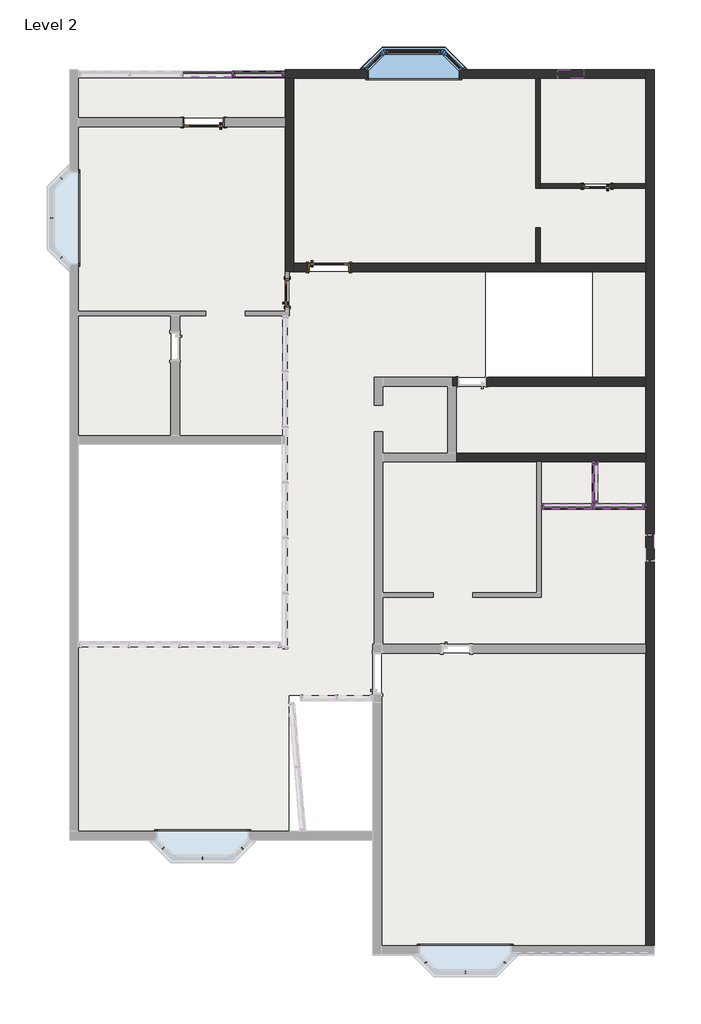
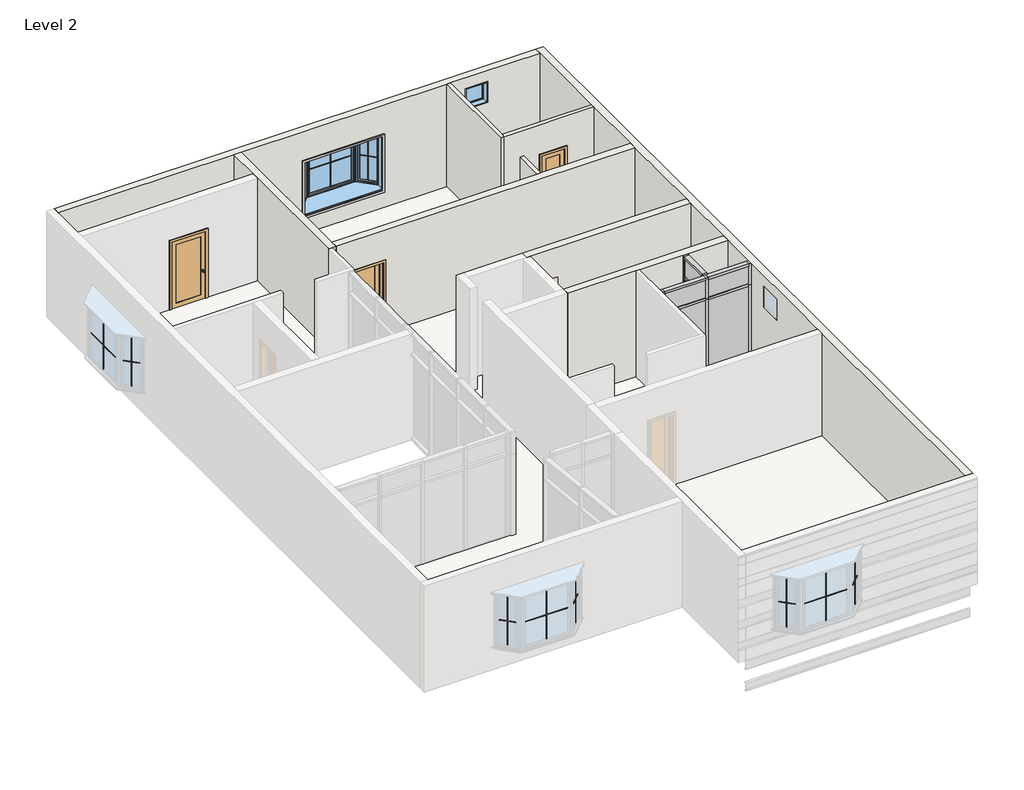
# One storey, part 5 of 5: 24 members, 16 proxies, 9 walls, 8 plates, 4 doors, 3 slabs, 2 windows.
"""IFC4 building model written with IfcOpenShell, lengths in millimetres."""

from ifc_helpers import new_model, si_unit, frame, origin, place, context, project, spatial, polyline, outline, extrude, faceted_brep, transform, mapped, element, save
from components import muntin_pattern_2x2_muntin_pattern_2x2_511ed329, muntin_pattern_2x2_muntin_pattern_2x2_63bd3b25, trim_window_interior_flat_picture_frame_e25f2530, door_interior_single_1_panel_wood_33af59b7, door_82825f5f, door_interior_single_1_panel_wood_secondary_door_3_x_7_9c4ddfbd, member_6e77e263, member_47bfaf8a, member_aaf6ec4e, member_7ce6cacc, member_f0fea5a5, member_ee409385, member_86adc6a2, member_92f44db0, member_11eb1482, member_fb055d8d, member_66f4a397, member_e9262278, system_panel_glazed_37c910ec, system_panel_glazed_3c79bf9a, system_panel_glazed_51086eaf, system_panel_glazed_73486e20, system_panel_glazed_4fbe648e, system_panel_glazed_a20b732f, window_6846e476, window_9f89e8e4

model = new_model("IFC4")

# Units and contexts
model_context = context("Model", 3, world=origin())
ifc_project = project(units=[si_unit("LENGTHUNIT", "METRE", prefix="MILLI")], contexts=[model_context])

# Site, building, storey
site = spatial("IfcSite", under=ifc_project)
building = spatial("IfcBuilding", under=site)
storey = spatial("IfcBuildingStorey", under=building, Name="Level 2", Elevation=3048.0)

# Proxies
placement = place(None, origin())
muntin_pattern_2x2_muntin_pattern_2x2_shape = muntin_pattern_2x2_muntin_pattern_2x2_511ed329(model_context)
element("IfcBuildingElementProxy", 1, Name="Muntin Pattern_2x2 : Muntin Pattern_2x2", ObjectType="Muntin Pattern_2x2 : Muntin Pattern_2x2", at=placement, inside=storey, context=model_context, shape_type="MappedRepresentation", body=[
    mapped(muntin_pattern_2x2_muntin_pattern_2x2_shape, transform((-41615.3380314, -10417.0163973, 3778.25), x_axis=(-1.0, 0.0, 0.0), y_axis=(0.0, -1.0, 0.0), z_axis=(0.0, 0.0, 1.0))),
])
element("IfcBuildingElementProxy", 2, Name="Muntin Pattern_2x2 : Muntin Pattern_2x2", ObjectType="Muntin Pattern_2x2 : Muntin Pattern_2x2", at=placement, inside=storey, context=model_context, shape_type="MappedRepresentation", body=[
    mapped(muntin_pattern_2x2_muntin_pattern_2x2_shape, transform((-42809.1380314, 10861.8336027, 3778.25), x_axis=(1.0, 0.0, 0.0), y_axis=(0.0, 1.0, 0.0), z_axis=(0.0, 0.0, 1.0))),
])
element("IfcBuildingElementProxy", 3, Name="Muntin Pattern_2x2 : Muntin Pattern_2x2", ObjectType="Muntin Pattern_2x2 : Muntin Pattern_2x2", at=placement, inside=storey, context=model_context, shape_type="MappedRepresentation", body=[
    mapped(muntin_pattern_2x2_muntin_pattern_2x2_shape, transform((-51175.2630314, 7016.9086027, 3778.25), x_axis=(0.0, 1.0, 0.0), y_axis=(-1.0, 0.0, 0.0), z_axis=(0.0, 0.0, 1.0))),
])
element("IfcBuildingElementProxy", 4, Name="Muntin Pattern_2x2 : Muntin Pattern_2x2", ObjectType="Muntin Pattern_2x2 : Muntin Pattern_2x2", at=placement, inside=storey, context=model_context, shape_type="MappedRepresentation", body=[
    mapped(muntin_pattern_2x2_muntin_pattern_2x2_shape, transform((-47685.9380314, -7775.4163973, 3778.25), x_axis=(-1.0, 0.0, 0.0), y_axis=(0.0, -1.0, 0.0), z_axis=(0.0, 0.0, 1.0))),
])
muntin_pattern_2x2_muntin_pattern_2x2_2_shape = muntin_pattern_2x2_muntin_pattern_2x2_63bd3b25(model_context)
element("IfcBuildingElementProxy", 5, Name="Muntin Pattern_2x2 : Muntin Pattern_2x2", ObjectType="Muntin Pattern_2x2 : Muntin Pattern_2x2", at=placement, inside=storey, context=model_context, shape_type="MappedRepresentation", body=[
    mapped(muntin_pattern_2x2_muntin_pattern_2x2_2_shape, transform((-40700.6463026, -10189.1206929, 3778.25), x_axis=(-0.7071067811865506, -0.7071067811865447, 0.0), y_axis=(0.7071067811865447, -0.7071067811865506, 0.0), z_axis=(0.0, 0.0, 1.0))),
])
element("IfcBuildingElementProxy", 6, Name="Muntin Pattern_2x2 : Muntin Pattern_2x2", ObjectType="Muntin Pattern_2x2 : Muntin Pattern_2x2", at=placement, inside=storey, context=model_context, shape_type="MappedRepresentation", body=[
    mapped(muntin_pattern_2x2_muntin_pattern_2x2_2_shape, transform((-42530.0297602, -10189.1206929, 3778.25), x_axis=(-0.7071067811865459, 0.7071067811865492, 0.0), y_axis=(-0.7071067811865492, -0.7071067811865459, 0.0), z_axis=(0.0, 0.0, 1.0))),
])
element("IfcBuildingElementProxy", 7, Name="Muntin Pattern_2x2 : Muntin Pattern_2x2", ObjectType="Muntin Pattern_2x2 : Muntin Pattern_2x2", at=placement, inside=storey, context=model_context, shape_type="MappedRepresentation", body=[
    mapped(muntin_pattern_2x2_muntin_pattern_2x2_2_shape, transform((-43723.8297602, 10633.9378984, 3778.25), x_axis=(0.7071067811865505, 0.7071067811865448, 0.0), y_axis=(-0.7071067811865448, 0.7071067811865505, 0.0), z_axis=(0.0, 0.0, 1.0))),
])
element("IfcBuildingElementProxy", 8, Name="Muntin Pattern_2x2 : Muntin Pattern_2x2", ObjectType="Muntin Pattern_2x2 : Muntin Pattern_2x2", at=placement, inside=storey, context=model_context, shape_type="MappedRepresentation", body=[
    mapped(muntin_pattern_2x2_muntin_pattern_2x2_2_shape, transform((-41894.4463026, 10633.9378984, 3778.25), x_axis=(0.707106781186546, -0.7071067811865491, 0.0), y_axis=(0.7071067811865491, 0.707106781186546, 0.0), z_axis=(0.0, 0.0, 1.0))),
])
element("IfcBuildingElementProxy", 9, Name="Muntin Pattern_2x2 : Muntin Pattern_2x2", ObjectType="Muntin Pattern_2x2 : Muntin Pattern_2x2", at=placement, inside=storey, context=model_context, shape_type="MappedRepresentation", body=[
    mapped(muntin_pattern_2x2_muntin_pattern_2x2_2_shape, transform((-50947.3673271, 6102.2168739, 3778.25), x_axis=(-0.707106781186546, 0.7071067811865492, 0.0), y_axis=(-0.7071067811865492, -0.707106781186546, 0.0), z_axis=(0.0, 0.0, 1.0))),
])
element("IfcBuildingElementProxy", 10, Name="Muntin Pattern_2x2 : Muntin Pattern_2x2", ObjectType="Muntin Pattern_2x2 : Muntin Pattern_2x2", at=placement, inside=storey, context=model_context, shape_type="MappedRepresentation", body=[
    mapped(muntin_pattern_2x2_muntin_pattern_2x2_2_shape, transform((-50947.3673271, 7931.6003316, 3778.25), x_axis=(0.7071067811865479, 0.7071067811865472, 0.0), y_axis=(-0.7071067811865472, 0.7071067811865479, 0.0), z_axis=(0.0, 0.0, 1.0))),
])
element("IfcBuildingElementProxy", 11, Name="Muntin Pattern_2x2 : Muntin Pattern_2x2", ObjectType="Muntin Pattern_2x2 : Muntin Pattern_2x2", at=placement, inside=storey, context=model_context, shape_type="MappedRepresentation", body=[
    mapped(muntin_pattern_2x2_muntin_pattern_2x2_2_shape, transform((-46771.2463026, -7547.5206929, 3778.25), x_axis=(-0.7071067811865506, -0.7071067811865447, 0.0), y_axis=(0.7071067811865447, -0.7071067811865506, 0.0), z_axis=(0.0, 0.0, 1.0))),
])
element("IfcBuildingElementProxy", 12, Name="Muntin Pattern_2x2 : Muntin Pattern_2x2", ObjectType="Muntin Pattern_2x2 : Muntin Pattern_2x2", at=placement, inside=storey, context=model_context, shape_type="MappedRepresentation", body=[
    mapped(muntin_pattern_2x2_muntin_pattern_2x2_2_shape, transform((-48600.6297602, -7547.5206929, 3778.25), x_axis=(-0.7071067811865459, 0.7071067811865492, 0.0), y_axis=(-0.7071067811865492, -0.7071067811865459, 0.0), z_axis=(0.0, 0.0, 1.0))),
])
trim_window_interior_flat_picture_frame_shape = trim_window_interior_flat_picture_frame_e25f2530(model_context)
element("IfcBuildingElementProxy", 13, Name="Trim-Window-Interior-Flat : Picture Frame", ObjectType="Trim-Window-Interior-Flat : Picture Frame", at=placement, inside=storey, context=model_context, shape_type="MappedRepresentation", body=[
    mapped(trim_window_interior_flat_picture_frame_shape, transform((-41615.3380314, -9797.8913973, 5232.4), x_axis=(-1.0, 0.0, 0.0), y_axis=(0.0, 0.0, 1.0), z_axis=(0.0, 1.0, 0.0))),
])
element("IfcBuildingElementProxy", 14, Name="Trim-Window-Interior-Flat : Picture Frame", ObjectType="Trim-Window-Interior-Flat : Picture Frame", at=placement, inside=storey, context=model_context, shape_type="MappedRepresentation", body=[
    mapped(trim_window_interior_flat_picture_frame_shape, transform((-42809.1380314, 10242.7086027, 5232.4), x_axis=(1.0, 0.0, 0.0), y_axis=(0.0, 0.0, 1.0), z_axis=(0.0, -1.0, 0.0))),
])
element("IfcBuildingElementProxy", 15, Name="Trim-Window-Interior-Flat : Picture Frame", ObjectType="Trim-Window-Interior-Flat : Picture Frame", at=placement, inside=storey, context=model_context, shape_type="MappedRepresentation", body=[
    mapped(trim_window_interior_flat_picture_frame_shape, transform((-50556.1380314, 7016.9086027, 5232.4), x_axis=(0.0, 1.0, 0.0), y_axis=(0.0, 0.0, 1.0), z_axis=(1.0, 0.0, 0.0))),
])
element("IfcBuildingElementProxy", 16, Name="Trim-Window-Interior-Flat : Picture Frame", ObjectType="Trim-Window-Interior-Flat : Picture Frame", at=placement, inside=storey, context=model_context, shape_type="MappedRepresentation", body=[
    mapped(trim_window_interior_flat_picture_frame_shape, transform((-47685.9380314, -7156.2913973, 5232.4), x_axis=(-1.0, 0.0, 0.0), y_axis=(0.0, 0.0, 1.0), z_axis=(0.0, 1.0, 0.0))),
])

# Doors
door_interior_single_1_panel_wood_shape = door_interior_single_1_panel_wood_33af59b7(model_context)
element("IfcDoor", 17, ObjectType="Door-Interior-Single-1_Panel-Wood", at=placement, inside=storey, context=model_context, shape_type="MappedRepresentation", body=[
    mapped(door_interior_single_1_panel_wood_shape, transform((-45733.3130314, 5289.7086027, 3048.0), x_axis=(0.0, 1.0, 0.0), y_axis=(-1.0, 0.0, 0.0), z_axis=(0.0, 0.0, 1.0))),
])
element("IfcDoor", 18, ObjectType="Door-Interior-Single-1_Panel-Wood", at=placement, inside=storey, context=model_context, shape_type="MappedRepresentation", body=[
    mapped(door_interior_single_1_panel_wood_shape, transform((-38567.3380314, 7750.3336027, 3048.0), x_axis=(-1.0, 0.0, 0.0), y_axis=(0.0, -1.0, 0.0), z_axis=(0.0, 0.0, 1.0))),
])
door_shape = door_82825f5f(model_context)
element("IfcDoor", 19, ObjectType="Door-Interior-Single-1_Panel-Wood : 36\" x 80\"", at=placement, inside=storey, context=model_context, shape_type="MappedRepresentation", body=[
    mapped(door_shape, transform((-47660.5380314, 9223.5336027, 3048.0), x_axis=(-1.0, 0.0, 0.0), y_axis=(0.0, -1.0, 0.0), z_axis=(0.0, 0.0, 1.0))),
])
door_interior_single_1_panel_wood_secondary_door_3_x_7_shape = door_interior_single_1_panel_wood_secondary_door_3_x_7_9c4ddfbd(model_context)
element("IfcDoor", 20, ObjectType="Door-Interior-Single-1_Panel-Wood : SECONDARY DOOR 3' X 7'", at=placement, inside=storey, context=model_context, shape_type="MappedRepresentation", body=[
    mapped(door_interior_single_1_panel_wood_secondary_door_3_x_7_shape, transform((-44764.9380314, 5877.0836027, 3048.0), x_axis=(1.0, 0.0, 0.0), y_axis=(0.0, 1.0, 0.0), z_axis=(0.0, 0.0, 1.0))),
])

# Members
member_shape = member_6e77e263(model_context)
element("IfcMember", 21, ObjectType="Rectangular Mullion : 2.5\" x 5\" rectangular", at=placement, inside=storey, context=model_context, shape_type="MappedRepresentation", body=[
    mapped(member_shape, transform((-38656.2380314, 354.3957124, 5486.4), x_axis=(1.0, 0.0, 0.0), y_axis=(0.0, -1.0, 0.0), z_axis=(0.0, 0.0, -1.0))),
])
member_2_shape = member_47bfaf8a(model_context)
element("IfcMember", 22, ObjectType="Rectangular Mullion : 2.5\" x 5\" rectangular", at=placement, inside=storey, context=model_context, shape_type="MappedRepresentation", body=[
    mapped(member_2_shape, transform((-39862.7380314, 354.3957124, 6096.0), x_axis=(-1.0, 0.0, 0.0), y_axis=(0.0, -1.0, 0.0), z_axis=(0.0, 0.0, 1.0))),
])
element("IfcMember", 23, ObjectType="Rectangular Mullion : 2.5\" x 5\" rectangular", at=placement, inside=storey, context=model_context, shape_type="MappedRepresentation", body=[
    mapped(member_2_shape, transform((-37449.7380314, 354.3957124, 5486.4), x_axis=(1.0, 0.0, 0.0), y_axis=(0.0, -1.0, 0.0), z_axis=(0.0, 0.0, -1.0))),
])
member_3_shape = member_aaf6ec4e(model_context)
element("IfcMember", 24, ObjectType="Rectangular Mullion : 2.5\" x 5\" rectangular", at=placement, inside=storey, context=model_context, shape_type="MappedRepresentation", body=[
    mapped(member_3_shape, transform((-37513.2380314, 354.3957124, 6096.0), x_axis=(0.0, 0.0, 1.0), y_axis=(0.0, -1.0, 0.0), z_axis=(1.0, 0.0, 0.0))),
])
element("IfcMember", 25, ObjectType="Rectangular Mullion : 2.5\" x 5\" rectangular", at=placement, inside=storey, context=model_context, shape_type="MappedRepresentation", body=[
    mapped(member_3_shape, transform((-38687.9880314, 354.3957124, 6096.0), x_axis=(0.0, 0.0, 1.0), y_axis=(0.0, -1.0, 0.0), z_axis=(1.0, 0.0, 0.0))),
])
element("IfcMember", 26, ObjectType="Rectangular Mullion : 2.5\" x 5\" rectangular", at=placement, inside=storey, context=model_context, shape_type="MappedRepresentation", body=[
    mapped(member_3_shape, transform((-39799.2380314, 354.3957124, 3048.0), x_axis=(0.0, 0.0, -1.0), y_axis=(0.0, -1.0, 0.0), z_axis=(-1.0, 0.0, 0.0))),
])
element("IfcMember", 27, ObjectType="Rectangular Mullion : 2.5\" x 5\" rectangular", at=placement, inside=storey, context=model_context, shape_type="MappedRepresentation", body=[
    mapped(member_3_shape, transform((-38624.4880314, 354.3957124, 3048.0), x_axis=(0.0, 0.0, -1.0), y_axis=(0.0, -1.0, 0.0), z_axis=(-1.0, 0.0, 0.0))),
])
member_4_shape = member_7ce6cacc(model_context)
element("IfcMember", 28, ObjectType="Rectangular Mullion : 2.5\" x 5\" rectangular", at=placement, inside=storey, context=model_context, shape_type="MappedRepresentation", body=[
    mapped(member_4_shape, transform((-38687.9880314, 354.3957124, 5486.4), x_axis=(0.0, 0.0, 1.0), y_axis=(0.0, -1.0, 0.0), z_axis=(1.0, 0.0, 0.0))),
])
element("IfcMember", 29, ObjectType="Rectangular Mullion : 2.5\" x 5\" rectangular", at=placement, inside=storey, context=model_context, shape_type="MappedRepresentation", body=[
    mapped(member_4_shape, transform((-37513.2380314, 354.3957124, 5486.4), x_axis=(0.0, 0.0, 1.0), y_axis=(0.0, -1.0, 0.0), z_axis=(1.0, 0.0, 0.0))),
])
member_5_shape = member_f0fea5a5(model_context)
element("IfcMember", 30, ObjectType="Rectangular Mullion : 2.5\" x 5\" rectangular", at=placement, inside=storey, context=model_context, shape_type="MappedRepresentation", body=[
    mapped(member_5_shape, transform((-38656.2380314, 354.3957124, 3048.0), x_axis=(1.0, 0.0, 0.0), y_axis=(0.0, -1.0, 0.0), z_axis=(0.0, 0.0, -1.0))),
])
member_6_shape = member_ee409385(model_context)
element("IfcMember", 31, ObjectType="Rectangular Mullion : 2.5\" x 5\" rectangular", at=placement, inside=storey, context=model_context, shape_type="MappedRepresentation", body=[
    mapped(member_6_shape, transform((-37449.7380314, 354.3957124, 3048.0), x_axis=(1.0, 0.0, 0.0), y_axis=(0.0, -1.0, 0.0), z_axis=(0.0, 0.0, -1.0))),
])
element("IfcMember", 32, ObjectType="Rectangular Mullion : 2.5\" x 5\" rectangular", at=placement, inside=storey, context=model_context, shape_type="MappedRepresentation", body=[
    mapped(member_6_shape, transform((-39862.7380314, 354.3957124, 5486.4), x_axis=(-1.0, 0.0, 0.0), y_axis=(0.0, -1.0, 0.0), z_axis=(0.0, 0.0, 1.0))),
])
element("IfcMember", 33, ObjectType="Rectangular Mullion : 2.5\" x 5\" rectangular", at=placement, inside=storey, context=model_context, shape_type="MappedRepresentation", body=[
    mapped(member_6_shape, transform((-38618.1380314, 1378.1086027, 3048.0), x_axis=(0.0, 1.0, 0.0), y_axis=(1.0, 0.0, 0.0), z_axis=(0.0, 0.0, -1.0))),
])
element("IfcMember", 34, ObjectType="Rectangular Mullion : 2.5\" x 5\" rectangular", at=placement, inside=storey, context=model_context, shape_type="MappedRepresentation", body=[
    mapped(member_2_shape, transform((-38618.1380314, 412.9086027, 6096.0), x_axis=(0.0, -1.0, 0.0), y_axis=(1.0, 0.0, 0.0), z_axis=(0.0, 0.0, 1.0))),
])
element("IfcMember", 35, ObjectType="Rectangular Mullion : 2.5\" x 5\" rectangular", at=placement, inside=storey, context=model_context, shape_type="MappedRepresentation", body=[
    mapped(member_2_shape, transform((-38618.1380314, 1378.1086027, 5486.4), x_axis=(0.0, 1.0, 0.0), y_axis=(1.0, 0.0, 0.0), z_axis=(0.0, 0.0, -1.0))),
])
element("IfcMember", 36, ObjectType="Rectangular Mullion : 2.5\" x 5\" rectangular", at=placement, inside=storey, context=model_context, shape_type="MappedRepresentation", body=[
    mapped(member_6_shape, transform((-38618.1380314, 412.9086027, 5486.4), x_axis=(0.0, -1.0, 0.0), y_axis=(1.0, 0.0, 0.0), z_axis=(0.0, 0.0, 1.0))),
])
member_7_shape = member_86adc6a2(model_context)
element("IfcMember", 37, ObjectType="Rectangular Mullion : 2.5\" x 5\" rectangular", at=placement, inside=storey, context=model_context, shape_type="MappedRepresentation", body=[
    mapped(member_7_shape, transform((-38618.1380314, 1314.6086027, 6096.0), x_axis=(0.0, 0.0, 1.0), y_axis=(1.0, 0.0, 0.0), z_axis=(0.0, 1.0, 0.0))),
])
element("IfcMember", 38, ObjectType="Rectangular Mullion : 2.5\" x 5\" rectangular", at=placement, inside=storey, context=model_context, shape_type="MappedRepresentation", body=[
    mapped(member_7_shape, transform((-38618.1380314, 476.4086027, 3048.0), x_axis=(0.0, 0.0, -1.0), y_axis=(1.0, 0.0, 0.0), z_axis=(0.0, -1.0, 0.0))),
])
member_8_shape = member_92f44db0(model_context)
element("IfcMember", 39, ObjectType="Rectangular Mullion : 2.5\" x 5\" rectangular", at=placement, inside=storey, context=model_context, shape_type="MappedRepresentation", body=[
    mapped(member_8_shape, transform((-38618.1380314, 1314.6086027, 5486.4), x_axis=(0.0, 0.0, 1.0), y_axis=(1.0, 0.0, 0.0), z_axis=(0.0, 1.0, 0.0))),
])
member_9_shape = member_11eb1482(model_context)
element("IfcMember", 40, ObjectType="Rectangular Mullion : 2.5\" x 5\" rectangular", at=placement, inside=storey, context=model_context, shape_type="MappedRepresentation", body=[
    mapped(member_9_shape, transform((-45844.4380314, 10344.3086027, 5209.4673659), x_axis=(0.0, 0.0, 1.0), y_axis=(0.0, -1.0, 0.0), z_axis=(1.0, 0.0, 0.0))),
])
member_10_shape = member_fb055d8d(model_context)
element("IfcMember", 41, ObjectType="Rectangular Mullion : 2.5\" x 5\" rectangular", at=placement, inside=storey, context=model_context, shape_type="MappedRepresentation", body=[
    mapped(member_10_shape, transform((-47006.4880316, 10344.3086027, 5209.4673659), x_axis=(0.0, 0.0, 1.0), y_axis=(0.0, -1.0, 0.0), z_axis=(1.0, 0.0, 0.0))),
])
element("IfcMember", 42, ObjectType="Rectangular Mullion : 2.5\" x 5\" rectangular", at=placement, inside=storey, context=model_context, shape_type="MappedRepresentation", body=[
    mapped(member_9_shape, transform((-46942.9880316, 10344.3086027, 3048.0), x_axis=(0.0, 0.0, -1.0), y_axis=(0.0, -1.0, 0.0), z_axis=(-1.0, 0.0, 0.0))),
])
member_11_shape = member_66f4a397(model_context)
element("IfcMember", 43, ObjectType="Rectangular Mullion : 2.5\" x 5\" rectangular", at=placement, inside=storey, context=model_context, shape_type="MappedRepresentation", body=[
    mapped(member_11_shape, transform((-46974.7380316, 10344.3086027, 3048.0), x_axis=(1.0, 0.0, 0.0), y_axis=(0.0, -1.0, 0.0), z_axis=(0.0, 0.0, -1.0))),
])
member_12_shape = member_e9262278(model_context)
element("IfcMember", 44, ObjectType="Rectangular Mullion : 2.5\" x 5\" rectangular", at=placement, inside=storey, context=model_context, shape_type="MappedRepresentation", body=[
    mapped(member_12_shape, transform((-45780.9380314, 10344.3086027, 3048.0), x_axis=(1.0, 0.0, 0.0), y_axis=(0.0, -1.0, 0.0), z_axis=(0.0, 0.0, -1.0))),
])

# Plates
system_panel_glazed_shape = system_panel_glazed_37c910ec(model_context)
element("IfcPlate", 45, ObjectType="System Panel : Glazed", at=placement, inside=storey, context=model_context, shape_type="MappedRepresentation", body=[
    mapped(system_panel_glazed_shape, transform((-39243.6130314, 354.3957124, 3111.5), x_axis=(1.0, 0.0, 0.0), y_axis=(0.0, 1.0, 0.0), z_axis=(0.0, 0.0, 1.0))),
])
element("IfcPlate", 46, ObjectType="System Panel : Glazed", at=placement, inside=storey, context=model_context, shape_type="MappedRepresentation", body=[
    mapped(system_panel_glazed_shape, transform((-38068.8630314, 354.3957124, 3111.5), x_axis=(1.0, 0.0, 0.0), y_axis=(0.0, 1.0, 0.0), z_axis=(0.0, 0.0, 1.0))),
])
system_panel_glazed_2_shape = system_panel_glazed_3c79bf9a(model_context)
element("IfcPlate", 47, ObjectType="System Panel : Glazed", at=placement, inside=storey, context=model_context, shape_type="MappedRepresentation", body=[
    mapped(system_panel_glazed_2_shape, transform((-39243.6130314, 354.3957124, 5518.15), x_axis=(1.0, 0.0, 0.0), y_axis=(0.0, 1.0, 0.0), z_axis=(0.0, 0.0, 1.0))),
])
element("IfcPlate", 48, ObjectType="System Panel : Glazed", at=placement, inside=storey, context=model_context, shape_type="MappedRepresentation", body=[
    mapped(system_panel_glazed_2_shape, transform((-38068.8630314, 354.3957124, 5518.15), x_axis=(1.0, 0.0, 0.0), y_axis=(0.0, 1.0, 0.0), z_axis=(0.0, 0.0, 1.0))),
])
system_panel_glazed_3_shape = system_panel_glazed_51086eaf(model_context)
element("IfcPlate", 49, ObjectType="System Panel : Glazed", at=placement, inside=storey, context=model_context, shape_type="MappedRepresentation", body=[
    mapped(system_panel_glazed_3_shape, transform((-38618.1380314, 895.5086027, 3111.5), x_axis=(0.0, 1.0, 0.0), y_axis=(-1.0, 0.0, 0.0), z_axis=(0.0, 0.0, 1.0))),
])
system_panel_glazed_4_shape = system_panel_glazed_73486e20(model_context)
element("IfcPlate", 50, ObjectType="System Panel : Glazed", at=placement, inside=storey, context=model_context, shape_type="MappedRepresentation", body=[
    mapped(system_panel_glazed_4_shape, transform((-38618.1380314, 895.5086027, 5518.15), x_axis=(0.0, 1.0, 0.0), y_axis=(-1.0, 0.0, 0.0), z_axis=(0.0, 0.0, 1.0))),
])
system_panel_glazed_5_shape = system_panel_glazed_4fbe648e(model_context)
element("IfcPlate", 51, ObjectType="System Panel : Glazed", at=placement, inside=storey, context=model_context, shape_type="MappedRepresentation", body=[
    mapped(system_panel_glazed_5_shape, transform((-46393.7130315, 10344.3086027, 3111.5), x_axis=(1.0, 0.0, 0.0), y_axis=(0.0, 1.0, 0.0), z_axis=(0.0, 0.0, 1.0))),
])
system_panel_glazed_6_shape = system_panel_glazed_a20b732f(model_context)
element("IfcPlate", 52, ObjectType="System Panel : Glazed", at=placement, inside=storey, context=model_context, shape_type="MappedRepresentation", body=[
    mapped(system_panel_glazed_6_shape, transform((-47571.6380315, 10344.3086027, 3111.5), x_axis=(1.0, 0.0, 0.0), y_axis=(0.0, 1.0, 0.0), z_axis=(0.0, 0.0, 1.0))),
])

# Slabs
element("IfcSlab", 53, ObjectType="MARBLE FLOORING 6\"", at=placement, inside=storey, context=model_context, shape_type="SweptSolid", body=[
    extrude(outline(polyline([(-45780.9380314, 10242.7086027), (-45780.9380314, 9328.3086027), (-50556.1380314, 9328.3086027), (-50556.1380314, 10242.7086027), (-45780.9380314, 10242.7086027)])), frame((0.0, 0.0, 2997.2), z_axis=(0.0, 0.0, 1.0), x_axis=(1.0, 0.0, 0.0)), (0.0, 0.0, 1.0), 152.4),
    extrude(outline(polyline([(-48422.5380314, 4756.3086027), (-48422.5380314, 1987.7086027), (-50556.1380314, 1987.7086027), (-50556.1380314, 4756.3086027), (-48422.5380314, 4756.3086027)])), frame((0.0, 0.0, 2997.2), z_axis=(0.0, 0.0, 1.0), x_axis=(1.0, 0.0, 0.0)), (0.0, 0.0, 1.0), 152.4),
    extrude(outline(polyline([(-37449.7380314, -3041.4913973), (-37449.7380314, -9797.8913973), (-43545.7380314, -9797.8913973), (-43545.7380314, -3041.4913973), (-37449.7380314, -3041.4913973)])), frame((0.0, 0.0, 2997.2), z_axis=(0.0, 0.0, 1.0), x_axis=(1.0, 0.0, 0.0)), (0.0, 0.0, 1.0), 152.4),
    extrude(outline(polyline([(-37449.7380314, 3130.7086027), (-37449.7380314, 1581.3086027), (-41818.5380314, 1581.3086027), (-41818.5380314, 3130.7086027), (-37449.7380314, 3130.7086027)])), frame((0.0, 0.0, 2997.2), z_axis=(0.0, 0.0, 1.0), x_axis=(1.0, 0.0, 0.0)), (0.0, 0.0, 1.0), 152.4),
    extrude(outline(polyline([(-50556.1380314, -2901.7913973), (-45882.5380314, -2901.7913973), (-45844.4380314, -2901.7913973), (-45844.4380314, -2939.8913973), (-45717.4380314, -2939.8913973), (-45717.4380314, 4756.3086027), (-45679.3380314, 4756.3086027), (-45679.3380314, 5772.3086027), (-41148.2472477, 5772.3086027), (-41148.2472477, 3333.9086027), (-43723.5380314, 3333.9086027), (-43723.5380314, 2686.2086027), (-43520.3380314, 2686.2086027), (-43520.3380314, 3130.7086027), (-42021.7380314, 3130.7086027), (-42021.7380314, 1581.3086027), (-43520.3380314, 1581.3086027), (-43520.3380314, 2076.6086027), (-43723.5380314, 2076.6086027), (-43723.5380314, -2838.2913973), (-43748.9380314, -2838.2913973), (-43748.9380314, -4017.5930974), (-45692.0380314, -4017.5930974), (-45692.0380314, -7156.2913973), (-50556.1380314, -7156.2913973), (-50556.1380314, -2901.7913973)])), frame((0.0, 0.0, 2997.2), z_axis=(0.0, 0.0, 1.0), x_axis=(1.0, 0.0, 0.0)), (0.0, 0.0, 1.0), 152.4),
])
element("IfcSlab", 54, ObjectType="MARBLE FLOORING 6\"", at=placement, inside=storey, context=model_context, shape_type="SweptSolid", body=[
    extrude(outline(polyline([(-45577.7380314, 5975.5086027), (-45577.7380314, 10242.7086027), (-39989.7380314, 10242.7086027), (-39989.7380314, 7702.7086027), (-37449.7380314, 7702.7086027), (-37449.7380314, 5975.5086027), (-39888.1380314, 5975.5086027), (-39888.1380314, 6788.3086027), (-39989.7380314, 6788.3086027), (-39989.7380314, 5975.5086027), (-45577.7380314, 5975.5086027)])), frame((0.0, 0.0, 2997.2), z_axis=(0.0, 0.0, 1.0), x_axis=(1.0, 0.0, 0.0)), (0.0, 0.0, 1.0), 152.4),
    extrude(outline(polyline([(-37449.7380314, 10242.7086027), (-37449.7380314, 7804.3086027), (-39888.1380314, 7804.3086027), (-39888.1380314, 10242.7086027), (-37449.7380314, 10242.7086027)])), frame((0.0, 0.0, 2997.2), z_axis=(0.0, 0.0, 1.0), x_axis=(1.0, 0.0, 0.0)), (0.0, 0.0, 1.0), 152.4),
    extrude(outline(polyline([(-45844.4380314, 1987.7086027), (-48219.3380314, 1987.7086027), (-48219.3380314, 4756.3086027), (-47609.7380314, 4756.3086027), (-47609.7380314, 4857.9086027), (-50556.1380314, 4857.9086027), (-50556.1380314, 9125.1086027), (-45780.9380314, 9125.1086027), (-45780.9380314, 4857.9086027), (-46695.3380314, 4857.9086027), (-46695.3380314, 4756.3086027), (-45844.4380314, 4756.3086027), (-45844.4380314, 1987.7086027)])), frame((0.0, 0.0, 2997.2), z_axis=(0.0, 0.0, 1.0), x_axis=(1.0, 0.0, 0.0)), (0.0, 0.0, 1.0), 152.4),
])
element("IfcSlab", 55, ObjectType="MARBLE FLOORING 6\"", at=placement, inside=storey, context=model_context, shape_type="SweptSolid", body=[
    extrude(outline(polyline([(-43520.3380314, -1746.0913973), (-42351.9380314, -1746.0913973), (-42351.9380314, -1644.4913973), (-43520.3380314, -1644.4913973), (-43520.3380314, 1378.1086027), (-39964.3380314, 1378.1086027), (-39964.3380314, -1644.4913973), (-41437.5380314, -1644.4913973), (-41437.5380314, -1746.0913973), (-39862.7380314, -1746.0913973), (-39862.7380314, 290.8957124), (-37449.7380314, 290.8957124), (-37449.7380314, -2838.2913973), (-43520.3380314, -2838.2913973), (-43520.3380314, -1746.0913973)])), frame((0.0, 0.0, 2895.6), z_axis=(0.0, 0.0, 1.0), x_axis=(1.0, 0.0, 0.0)), (0.0, 0.0, 1.0), 152.4),
    extrude(outline(polyline([(-38681.6380314, 1378.1086027), (-38681.6380314, 412.9086027), (-39862.7380314, 412.9086027), (-39862.7380314, 1378.1086027), (-38681.6380314, 1378.1086027)])), frame((0.0, 0.0, 2895.6), z_axis=(0.0, 0.0, 1.0), x_axis=(1.0, 0.0, 0.0)), (0.0, 0.0, 1.0), 152.4),
    extrude(outline(polyline([(-37449.7380314, 1378.1086027), (-37449.7380314, 417.8957124), (-38554.6380314, 417.8957124), (-38554.6380314, 1378.1086027), (-37449.7380314, 1378.1086027)])), frame((0.0, 0.0, 2895.6), z_axis=(0.0, 0.0, 1.0), x_axis=(1.0, 0.0, 0.0)), (0.0, 0.0, 1.0), 152.4),
    extrude(outline(polyline([(-37449.7380314, 5772.3086027), (-37449.7380314, 3333.9086027), (-38668.9380314, 3333.9086027), (-38668.9380314, 5772.3086027), (-37449.7380314, 5772.3086027)])), frame((0.0, 0.0, 2895.6), z_axis=(0.0, 0.0, 1.0), x_axis=(1.0, 0.0, 0.0)), (0.0, 0.0, 1.0), 152.4),
])

# Walls
element("IfcWall", 56, ObjectType="INNER WALL 4\"", at=placement, inside=storey, context=model_context, shape_type="Brep", body=[
    faceted_brep([(-39989.7380314, 10242.7086027, 3048.0), (-39989.7380314, 7702.7086027, 3048.0), (-39989.7380314, 7702.7086027, 6096.0), (-39989.7380314, 10242.7086027, 6096.0), (-39888.1380314, 10242.7086027, 3048.0), (-39888.1380314, 10242.7086027, 6096.0), (-39888.1380314, 7804.3086027, 6096.0), (-39888.1380314, 7702.7086027, 6096.0), (-39888.1380314, 7702.7086027, 3048.0), (-39888.1380314, 7804.3086027, 3048.0)], [[[0, 1, 2, 3]], [[4, 5, 6, 7, 8, 9]], [[1, 0, 4, 9, 8]], [[3, 2, 7, 6, 5]], [[2, 1, 8, 7]], [[0, 3, 5, 4]]]),
])
element("IfcWall", 57, ObjectType="INNER WALL 4\"", at=placement, inside=storey, context=model_context, shape_type="SweptSolid", body=[
    extrude(outline(polyline([(6096.0, -37449.7380314), (6096.0, -39888.1380314), (3048.0, -39888.1380314), (3048.0, -38897.5380314), (5207.0, -38897.5380314), (5207.0, -38237.1380314), (3048.0, -38237.1380314), (3048.0, -37449.7380314), (6096.0, -37449.7380314)])), frame((0.0, 7702.7086027, 0.0), z_axis=(0.0, 1.0, 0.0), x_axis=(0.0, 0.0, 1.0)), (0.0, 0.0, 1.0), 101.6),
])
element("IfcWall", 58, ObjectType="INNER WALL 4\"", at=placement, inside=storey, context=model_context, shape_type="SweptSolid", body=[
    extrude(outline(polyline([(-39888.1380314, 6788.3086027), (-39888.1380314, 5975.5086027), (-39989.7380314, 5975.5086027), (-39989.7380314, 6788.3086027), (-39888.1380314, 6788.3086027)])), frame((0.0, 0.0, 3048.0), z_axis=(0.0, 0.0, 1.0), x_axis=(1.0, 0.0, 0.0)), (0.0, 0.0, 1.0), 3048.0),
])
element("IfcWall", 59, ObjectType="OUTER WALL 8\"", at=placement, inside=storey, context=model_context, shape_type="Brep", body=[
    faceted_brep([(-37246.5380314, -9797.8913973, 3048.0), (-37246.5380314, 10445.9086027, 3048.0), (-37246.5380314, 10445.9086027, 6096.0), (-37246.5380314, -9797.8913973, 6096.0), (-37246.5380314, -306.0042876, 5791.2), (-37246.5380314, -306.0042876, 5181.6), (-37246.5380314, -915.6042876, 5181.6), (-37246.5380314, -915.6042876, 5791.2), (-37449.7380314, -9797.8913973, 3048.0), (-37449.7380314, -9797.8913973, 6096.0), (-37449.7380314, -3041.4913973, 6096.0), (-37449.7380314, -2838.2913973, 6096.0), (-37449.7380314, 1378.1086027, 6096.0), (-37449.7380314, 1581.3086027, 6096.0), (-37449.7380314, 3130.7086027, 6096.0), (-37449.7380314, 3333.9086027, 6096.0), (-37449.7380314, 5772.3086027, 6096.0), (-37449.7380314, 5975.5086027, 6096.0), (-37449.7380314, 7702.7086027, 6096.0), (-37449.7380314, 7804.3086027, 6096.0), (-37449.7380314, 10242.7086027, 6096.0), (-37449.7380314, 10445.9086027, 6096.0), (-37449.7380314, 10445.9086027, 3048.0), (-37449.7380314, 10242.7086027, 3048.0), (-37449.7380314, 7804.3086027, 3048.0), (-37449.7380314, 7702.7086027, 3048.0), (-37449.7380314, 5975.5086027, 3048.0), (-37449.7380314, 5772.3086027, 3048.0), (-37449.7380314, 3333.9086027, 3048.0), (-37449.7380314, 3130.7086027, 3048.0), (-37449.7380314, 1581.3086027, 3048.0), (-37449.7380314, 1378.1086027, 3048.0), (-37449.7380314, -2838.2913973, 3048.0), (-37449.7380314, -3041.4913973, 3048.0), (-37449.7380314, -306.0042876, 5791.2), (-37449.7380314, -915.6042876, 5791.2), (-37449.7380314, -915.6042876, 5181.6), (-37449.7380314, -306.0042876, 5181.6)], [[[0, 1, 2, 3], [4, 5, 6, 7]], [[8, 9, 10, 11, 12, 13, 14, 15, 16, 17, 18, 19, 20, 21, 22, 23, 24, 25, 26, 27, 28, 29, 30, 31, 32, 33], [34, 35, 36, 37]], [[1, 0, 8, 33, 32, 31, 30, 29, 28, 27, 26, 25, 24, 23, 22]], [[3, 2, 21, 20, 19, 18, 17, 16, 15, 14, 13, 12, 11, 10, 9]], [[0, 3, 9, 8]], [[2, 1, 22, 21]], [[5, 4, 34, 37]], [[6, 5, 37, 36]], [[7, 6, 36, 35]], [[4, 7, 35, 34]]]),
])
element("IfcWall", 60, ObjectType="OUTER WALL 8\"", at=placement, inside=storey, context=model_context, shape_type="Brep", body=[
    faceted_brep([(-37449.7380314, 1581.3086027, 3048.0), (-41818.5380314, 1581.3086027, 3048.0), (-41818.5380314, 1581.3086027, 6096.0), (-37449.7380314, 1581.3086027, 6096.0), (-37449.7380314, 1378.1086027, 3048.0), (-37449.7380314, 1378.1086027, 6096.0), (-39862.7380314, 1378.1086027, 6096.0), (-39964.3380314, 1378.1086027, 6096.0), (-41818.5380314, 1378.1086027, 6096.0), (-41818.5380314, 1378.1086027, 3048.0), (-39964.3380314, 1378.1086027, 3048.0), (-39862.7380314, 1378.1086027, 3048.0)], [[[0, 1, 2, 3]], [[4, 5, 6, 7, 8, 9, 10, 11]], [[1, 0, 4, 11, 10, 9]], [[3, 2, 8, 7, 6, 5]], [[0, 3, 5, 4]], [[2, 1, 9, 8]]]),
])
element("IfcWall", 61, ObjectType="OUTER WALL 8\"", at=placement, inside=storey, context=model_context, shape_type="Brep", body=[
    faceted_brep([(-41920.1380314, 3333.9086027, 3048.0), (-41920.1380314, 3333.9086027, 6096.0), (-37449.7380314, 3333.9086027, 6096.0), (-37449.7380314, 3333.9086027, 3048.0), (-41132.7380314, 3333.9086027, 3048.0), (-41132.7380314, 3333.9086027, 5207.0), (-41793.1380314, 3333.9086027, 5207.0), (-41793.1380314, 3333.9086027, 3048.0), (-41920.1380314, 3130.7086027, 6096.0), (-41920.1380314, 3130.7086027, 3048.0), (-41818.5380314, 3130.7086027, 3048.0), (-41793.1380314, 3130.7086027, 3048.0), (-41793.1380314, 3130.7086027, 5207.0), (-41132.7380314, 3130.7086027, 5207.0), (-41132.7380314, 3130.7086027, 3048.0), (-37449.7380314, 3130.7086027, 3048.0), (-37449.7380314, 3130.7086027, 6096.0), (-41818.5380314, 3130.7086027, 6096.0)], [[[0, 1, 2, 3, 4, 5, 6, 7]], [[8, 9, 10, 11, 12, 13, 14, 15, 16, 17]], [[3, 15, 14, 4]], [[9, 0, 7, 11, 10]], [[1, 0, 9, 8]], [[2, 1, 8, 17, 16]], [[3, 2, 16, 15]], [[6, 12, 11, 7]], [[12, 6, 5, 13]], [[13, 5, 4, 14]]]),
])
element("IfcWall", 62, ObjectType="OUTER WALL 8\"", at=placement, inside=storey, context=model_context, shape_type="Brep", body=[
    faceted_brep([(-45780.9380314, 10242.7086027, 3048.0), (-45780.9380314, 9328.3086027, 3048.0), (-45780.9380314, 9125.1086027, 3048.0), (-45780.9380314, 5772.3086027, 3048.0), (-45780.9380314, 5772.3086027, 6096.0), (-45780.9380314, 9125.1086027, 6096.0), (-45780.9380314, 9328.3086027, 6096.0), (-45780.9380314, 10242.7086027, 6096.0), (-45577.7380314, 10242.7086027, 3048.0), (-45577.7380314, 10242.7086027, 6096.0), (-45577.7380314, 5975.5086027, 6096.0), (-45577.7380314, 5772.3086027, 6096.0), (-45577.7380314, 5772.3086027, 3048.0), (-45577.7380314, 5975.5086027, 3048.0), (-45679.3380314, 5772.3086027, 3048.0), (-45679.3380314, 5772.3086027, 6096.0)], [[[0, 1, 2, 3, 4, 5, 6, 7]], [[8, 9, 10, 11, 12, 13]], [[3, 2, 1, 0, 8, 13, 12, 14]], [[7, 6, 5, 4, 15, 11, 10, 9]], [[4, 3, 14, 12, 11, 15]], [[0, 7, 9, 8]]]),
])
element("IfcWall", 63, ObjectType="OUTER WALL 8\"", at=placement, inside=storey, context=model_context, shape_type="Brep", body=[
    faceted_brep([(-37449.7380314, 5772.3086027, 6096.0), (-45577.7380314, 5772.3086027, 6096.0), (-45577.7380314, 5772.3086027, 3048.0), (-45247.5380314, 5772.3086027, 3048.0), (-45247.5380314, 5772.3086027, 5207.0), (-44282.3380314, 5772.3086027, 5207.0), (-44282.3380314, 5772.3086027, 3048.0), (-37449.7380314, 5772.3086027, 3048.0), (-45577.7380314, 5975.5086027, 6096.0), (-39989.7380314, 5975.5086027, 6096.0), (-39888.1380314, 5975.5086027, 6096.0), (-37449.7380314, 5975.5086027, 6096.0), (-37449.7380314, 5975.5086027, 3048.0), (-39888.1380314, 5975.5086027, 3048.0), (-39989.7380314, 5975.5086027, 3048.0), (-44282.3380314, 5975.5086027, 3048.0), (-44282.3380314, 5975.5086027, 5207.0), (-45247.5380314, 5975.5086027, 5207.0), (-45247.5380314, 5975.5086027, 3048.0), (-45577.7380314, 5975.5086027, 3048.0)], [[[0, 1, 2, 3, 4, 5, 6, 7]], [[8, 9, 10, 11, 12, 13, 14, 15, 16, 17, 18, 19]], [[2, 19, 18, 3]], [[12, 7, 6, 15, 14, 13]], [[1, 0, 11, 10, 9, 8]], [[2, 1, 8, 19]], [[0, 7, 12, 11]], [[5, 16, 15, 6]], [[16, 5, 4, 17]], [[17, 4, 3, 18]]]),
])
element("IfcWall", 64, ObjectType="OUTER WALL 8\"", at=placement, inside=storey, context=model_context, shape_type="Brep", body=[
    faceted_brep([(-50556.1380314, 10445.9086027, 6096.0), (-37449.7380314, 10445.9086027, 6096.0), (-37449.7380314, 10445.9086027, 3048.0), (-45780.9380314, 10445.9086027, 3048.0), (-45780.9380314, 10445.9086027, 5209.4673659), (-50556.1380314, 10445.9086027, 5209.4673659), (-41692.9466227, 10445.9086027, 5232.4), (-43925.3294401, 10445.9086027, 5232.4), (-43925.3294401, 10445.9086027, 3657.6), (-41692.9466227, 10445.9086027, 3657.6), (-38872.1380314, 10445.9086027, 5791.2), (-39481.7380314, 10445.9086027, 5791.2), (-39481.7380314, 10445.9086027, 5181.6), (-38872.1380314, 10445.9086027, 5181.6), (-37449.7380314, 10242.7086027, 6096.0), (-39888.1380314, 10242.7086027, 6096.0), (-39989.7380314, 10242.7086027, 6096.0), (-45577.7380314, 10242.7086027, 6096.0), (-45780.9380314, 10242.7086027, 6096.0), (-50556.1380314, 10242.7086027, 6096.0), (-50556.1380314, 10242.7086027, 5209.4673659), (-45780.9380314, 10242.7086027, 5209.4673659), (-45780.9380314, 10242.7086027, 3048.0), (-45577.7380314, 10242.7086027, 3048.0), (-39989.7380314, 10242.7086027, 3048.0), (-39888.1380314, 10242.7086027, 3048.0), (-37449.7380314, 10242.7086027, 3048.0), (-43875.9380314, 10242.7086027, 5232.4), (-41742.3380314, 10242.7086027, 5232.4), (-41742.3380314, 10242.7086027, 3657.6), (-43875.9380314, 10242.7086027, 3657.6), (-38872.1380314, 10242.7086027, 5791.2), (-38872.1380314, 10242.7086027, 5181.6), (-39481.7380314, 10242.7086027, 5181.6), (-39481.7380314, 10242.7086027, 5791.2), (-43875.9380314, 10396.5171941, 5232.4), (-41742.3380314, 10396.5171941, 5232.4), (-43875.9380314, 10396.5171941, 3657.6), (-41742.3380314, 10396.5171941, 3657.6)], [[[0, 1, 2, 3, 4, 5], [6, 7, 8, 9], [10, 11, 12, 13]], [[14, 15, 16, 17, 18, 19, 20, 21, 22, 23, 24, 25, 26], [27, 28, 29, 30], [31, 32, 33, 34]], [[2, 26, 25, 24, 23, 22, 3]], [[1, 0, 19, 18, 17, 16, 15, 14]], [[2, 1, 14, 26]], [[19, 0, 5, 20]], [[4, 21, 20, 5]], [[21, 4, 3, 22]], [[35, 7, 6, 36, 28, 27]], [[37, 30, 29, 38, 9, 8]], [[35, 27, 30, 37]], [[28, 36, 38, 29]], [[36, 6, 9, 38]], [[7, 35, 37, 8]], [[32, 31, 10, 13]], [[33, 32, 13, 12]], [[34, 33, 12, 11]], [[31, 34, 11, 10]]]),
])

# Windows
window_shape = window_6846e476(model_context)
element("IfcWindow", 65, ObjectType="Fixed : 24\" x 24\"", at=placement, inside=storey, context=model_context, shape_type="MappedRepresentation", body=[
    mapped(window_shape, transform((-39138.8380314, 10344.3086027, 4267.2), x_axis=(1.0, 0.0, 0.0), y_axis=(0.0, 1.0, 0.0), z_axis=(0.0, 0.0, 1.0))),
])
window_2_shape = window_9f89e8e4(model_context)
element("IfcWindow", 66, ObjectType="Window-Bay-Casement-45_Degree_Angle : 84\" x 60\" x 18\"", at=placement, inside=storey, context=model_context, shape_type="MappedRepresentation", body=[
    mapped(window_2_shape, transform((-42809.1380314, 10344.3086027, 3048.0), x_axis=(1.0, 0.0, 0.0), y_axis=(0.0, 1.0, 0.0), z_axis=(0.0, 0.0, 1.0))),
])

save(model, "model.ifc")

# Revit data of these elements
# Type "Muntin Pattern_2x2 : Muntin Pattern_2x2"
#   Width [instance default] = 4' - 0"
#   Thickness = 0' - 0 1/2"
#   Height [instance default] = 4' - 0"
#   Distance = 0' - 0 3/4"
#   Interior Material [instance default] = none
#   Exterior Material [instance default] = none
#   Default Elevation = 0
# Type "Trim-Window-Interior-Flat : Picture Frame"
#   Trim Thickness_Picture Frame = 0' - 1 1/4"
#   Trim Width = 0' - 2 1/4"
#   Trim Thickness_with Sill = 0' - 0 3/4"
#   Sill Thickness = 0' - 1 1/4"
#   Opening Width [instance default] = 2' - 0"
#   Opening Height [instance default] = 3' - 0"
#   Default Elevation = 4' - 0"
#   Sill = no
#   Picture Frame = yes
#   Trim Material [instance default] = none
# Type "Door-Interior-Single-1_Panel-Wood"
#   Type Mark = "12"
#   Assembly Code = "C1020300"
#   Analytic Construction = "Wooden"
#   Top Rail = 0' - 4 11/16"
#   Thickness = 0' - 1 3/8"
#   Thermal Resistance (R) = 2.5876 (h·ft²·°F)/BTU
#   Swing Angle [instance default] = 90.00°
#   Stiles = 0' - 4 3/4"
#   Rough Width = 2' - 2"
#   Rough Height = 7' - 1"
#   Height = 7' - 0"
#   Width = 2' - 0"
#   Heat Transfer Coefficient (U) = 0.3865 BTU/(h·ft²·°F)
#   Bottom Rail = 0' - 9 1/8"
#   Trim Material = Cherry
#   Panel Material = Cherry
#   Frame Material = Cherry
#   Door Handle Material = Aluminum
#   Visual Light Transmittance = 0
#   Solar Heat Gain Coefficient = 0
#   Wall Closure = (empty or 0)
#   Function = (empty or 0)
# Type "Door-Interior-Single-1_Panel-Wood : 36\" x 80\""
#   Type Mark = "10"
#   Assembly Code = "C1020300"
#   Analytic Construction = "Wooden"
#   Top Rail = 0' - 4 11/16"
#   Thickness = 0' - 1 3/8"
#   Thermal Resistance (R) = 2.5876 (h·ft²·°F)/BTU
#   Swing Angle [instance default] = 90.00°
#   Stiles = 0' - 4 3/4"
#   Rough Width = 3' - 2"
#   Rough Height = 6' - 9"
#   Height = 6' - 8"
#   Width = 3' - 0"
#   Heat Transfer Coefficient (U) = 0.3865 BTU/(h·ft²·°F)
#   Bottom Rail = 0' - 9 1/8"
#   Trim Material = Cherry
#   Panel Material = Cherry
#   Frame Material = Cherry
#   Door Handle Material = Aluminum
#   Visual Light Transmittance = 0
#   Solar Heat Gain Coefficient = 0
#   Wall Closure = (empty or 0)
#   Function = (empty or 0)
# Type "Door-Interior-Single-1_Panel-Wood : SECONDARY DOOR 3' X 7'"
#   Type Mark = "11"
#   Assembly Code = "C1020300"
#   Analytic Construction = "Wooden"
#   Top Rail = 0' - 4 11/16"
#   Thickness = 0' - 1 3/8"
#   Thermal Resistance (R) = 2.5876 (h·ft²·°F)/BTU
#   Swing Angle [instance default] = 90.00°
#   Stiles = 0' - 4 3/4"
#   Rough Width = 3' - 2"
#   Rough Height = 7' - 1"
#   Height = 7' - 0"
#   Width = 3' - 0"
#   Heat Transfer Coefficient (U) = 0.3865 BTU/(h·ft²·°F)
#   Bottom Rail = 0' - 9 1/8"
#   Trim Material = Cherry
#   Panel Material = Cherry
#   Frame Material = Cherry
#   Door Handle Material = Aluminum
#   Visual Light Transmittance = 0
#   Solar Heat Gain Coefficient = 0
#   Wall Closure = (empty or 0)
#   Function = (empty or 0)
# Type "Rectangular Mullion : 2.5\" x 5\" rectangular"
#   built-in parameter 1007304 = 0.416667 (stored number, unit not read)
#   built-in parameter 1007301 = 0.104167 (stored number, unit not read)
#   built-in parameter 1007300 = 0.104167 (stored number, unit not read)
# Type "System Panel : Glazed"
#   Construction Type Id = "GSP4R"
#   Analytic Construction = "1/8 in Pilkington single glazing"
#   Visual Light Transmittance = 0.9
#   Solar Heat Gain Coefficient = 0.86
#   Heat Transfer Coefficient (U) = 1.18115 BTU/(h·ft²·°F)
#   Define Thermal Properties by = 1
# Type "MARBLE FLOORING 6\""
#   Assembly Code = "B1010"
#   Function = 0
#   Layers, outside or top first: 0' - 6" "MARBLE FLOOR" (function 1)
# Type "INNER WALL 4\""
#   Assembly Code = "B2010"
#   Layers, outside or top first: 0' - 4" "BEIGE COLOUR" (function 1)
# Type "OUTER WALL 8\""
#   Assembly Code = "B2010"
#   Layers, outside or top first: 0' - 8" "BEIGE COLOUR" (function 1)
# Type "Fixed : 24\" x 24\""
#   Type Mark = "3"
#   Construction Type Id = "GSP4R"
#   Assembly Code = "B2020100"
#   Analytic Construction = "1/8 in Pilkington single glazing"
#   Visual Light Transmittance = 0.9
#   Solar Heat Gain Coefficient = 0.78
#   Heat Transfer Coefficient (U) = 0.6496 BTU/(h·ft²·°F)
#   Height = 2' - 0"
#   Default Sill Height = 3' - 0"
#   Width = 2' - 0"
#   Window Inset = 0' - 0 3/4"
#   Define Thermal Properties by = 1
#   Define Thermal Properties by = 1
#   Glass Pane Material = Glass
#   Sash Material = Sash
#   Wall Closure = (empty or 0)
# Type "Window-Bay-Casement-45_Degree_Angle : 84\" x 60\" x 18\""
#   Type Mark = "18"
#   Fire Rating = "0.5h"
#   Assembly Code = "B2020100"
#   Analytic Construction = "Double glazing - domestic"
#   Width of Middle Sash = 4' - 2.38909"
#   Width = 7' - 0"
#   Visual Light Transmittance = 0.81
#   Thermal Resistance (R) = 1.8146 (h·ft²·°F)/BTU
#   Solar Heat Gain Coefficient = 0.76
#   Rough Width = 7' - 0 1/2"
#   Rough Height = 5' - 0 1/2"
#   Length 4 = 0' - 1.13909"
#   Length 3 = 0' - 0.51777"
#   Length 2 = 4' - 7.42462"
#   Length 1 = 1' - 2.80546"
#   Wall Thickness [instance default] = 0' - 6"
#   Trim Width = 7' - 5.03553"
#   Trim Height = 5' - 0"
#   Height 1 = 5' - 2"
#   Height = 5' - 0"
#   Heat Transfer Coefficient (U) = 0.5511 BTU/(h·ft²·°F)
#   Depth = 1' - 6"
#   Default Sill Height = 2' - 0"
#   Angle 1 = 22.50°
#   Angle = 45.00°
#   Center Muntin Visibility = yes
#   Side Muntin Visibility = yes
#   Interior Trim Visibility [instance default] = yes
#   Exterior Trim Visibility [instance default] = yes
#   Center Muntin Pattern = Muntin Pattern_2x2 : Muntin Pattern_2x2
#   Side Muntin Pattern = Muntin Pattern_2x2 : Muntin Pattern_2x2
#   Interior Trim Material = Wood - Stained
#   Exterior Trim Material = Clad - White
#   Exterior Trim = element 406231
#   Interior Trim = Trim-Window-Interior-Flat : Picture Frame
#   Interior Frame Material = Wood - Stained
#   Glass Panel Material = Glass
#   Exterior Frame Material = Clad - White
#   Wall Closure = (empty or 0)
# Elements 1, 2, 3, 4 (IfcBuildingElementProxy, "Muntin Pattern_2x2 : Muntin Pattern_2x2")
#   Width = 3' - 8.88909"
#   Height = 4' - 6 1/2"
#   Interior Material = Wood - Stained
#   Exterior Material = Clad - White
#   Phase Created = New Construction
#   Materials on its faces: "Clad - White", "Wood - Stained"
# Elements 5, 6, 7, 8, 9, 10, 11, 12 (IfcBuildingElementProxy, "Muntin Pattern_2x2 : Muntin Pattern_2x2")
#   Width = 1' - 4.18808"
#   Height = 4' - 6 1/2"
#   Interior Material = Wood - Stained
#   Exterior Material = Clad - White
#   Phase Created = New Construction
#   Materials on its faces: "Clad - White", "Wood - Stained"
# Elements 13, 14, 15, 16 (IfcBuildingElementProxy, "Trim-Window-Interior-Flat : Picture Frame")
#   Opening Width = 7' - 0"
#   Opening Height = 5' - 2"
#   Trim Material = Wood - Stained
#   Phase Created = New Construction
#   Materials on its faces: "Wood - Stained"
# Elements 17, 18 (IfcDoor, "Door-Interior-Single-1_Panel-Wood")
#   Swing Angle = 90.00°
#   Phase Created = New Construction
#   Materials on its faces: "Cherry", "Aluminum"
# Element 19 (IfcDoor, "Door-Interior-Single-1_Panel-Wood : 36\" x 80\"")
#   Swing Angle = 90.00°
#   Phase Created = New Construction
#   Materials on its faces: "Cherry", "Aluminum"
# Element 20 (IfcDoor, "Door-Interior-Single-1_Panel-Wood : SECONDARY DOOR 3' X 7'")
#   Swing Angle = 90.00°
#   Phase Created = New Construction
#   Materials on its faces: "Cherry", "Aluminum"
# Elements 21, 22, 23, 24, 25, 26, 27, 28, 29, 30, 31, 32, 33, 34, 35, 36, 37, 38, 39, 40, 41, 42, 43, 44 (IfcMember, "Rectangular Mullion : 2.5\" x 5\" rectangular")
#   Phase Created = New Construction
#   Materials on its faces: "Aluminum"
# Elements 45, 46, 47, 48, 49, 50, 51, 52 (IfcPlate, "System Panel : Glazed")
#   Phase Created = New Construction
#   Materials on its faces: "glass panel 223"
# Element 53 (IfcSlab, "MARBLE FLOORING 6\"")
#   Height Offset From Level = 0' - 4"
#   Phase Created = New Construction
#   Materials on its faces: "MARBLE FLOOR"
# Element 54 (IfcSlab, "MARBLE FLOORING 6\"")
#   built-in parameter 1001955 = -1.5708 (stored number, unit not read)
#   Height Offset From Level = 0' - 4"
#   Phase Created = New Construction
#   Materials on its faces: "MARBLE FLOOR"
# Element 55 (IfcSlab, "MARBLE FLOORING 6\"")
#   built-in parameter 1001955 = 1.5708 (stored number, unit not read)
#   Height Offset From Level = 0' - 0"
#   Phase Created = New Construction
#   Materials on its faces: "MARBLE FLOOR"
# Elements 56, 57, 58 (IfcWall, "INNER WALL 4\"")
#   Top Offset = 0' - 0"
#   Base Offset = 0' - 0"
#   wall height = 10' - 0"
#   Phase Created = New Construction
#   Base Constraint = Level 2
#   Top Constraint = Level 3
#   Materials on its faces: "BEIGE COLOUR"
# Elements 59, 60, 61, 62, 63, 64 (IfcWall, "OUTER WALL 8\"")
#   Top Offset = 0' - 0"
#   Base Offset = 0' - 0"
#   wall height = 10' - 0"
#   Phase Created = New Construction
#   Base Constraint = Level 2
#   Top Constraint = Level 3
#   Materials on its faces: "BEIGE COLOUR"
# Element 65 (IfcWindow, "Fixed : 24\" x 24\"")
#   Mark = "10"
#   Phase Created = New Construction
#   Materials on its faces: "Sash", "Glass"
# Element 66 (IfcWindow, "Window-Bay-Casement-45_Degree_Angle : 84\" x 60\" x 18\"")
#   Mark = "9"
#   Interior Trim Visibility = yes
#   Exterior Trim Visibility = yes
#   Phase Created = New Construction
#   Materials on its faces: "Wood - Stained", "Clad - White", "Glass"
# Materials
#   "Cherry": class "Wood", colour RGB 226 177 128, transparency 0, Description = "Prunus Serotina", Cost = 0
#   "Aluminum": class "Metal", colour RGB 247 247 247, transparency 0, Description = "Aluminum 6061", Cost = 0
#   "MARBLE FLOOR": class "Generic", colour RGB 120 120 120, transparency 0, Cost = 0
#   "BEIGE COLOUR": class "Generic", colour RGB 120 120 120, transparency 0, Cost = 0
#   "Glass": class "Glass", colour RGB 0 128 192, transparency 0.75, Description = "Soda Lime Glass", Cost = 0
#   "Sash": class "Wood", colour RGB 224 178 126, transparency 0, Cost = 0
#   "Wood - Stained": class "Wood", colour RGB 224 178 126, transparency 0, Cost = 0
#   "Clad - White": class "Wood", colour RGB 242 242 238, transparency 0, Cost = 0
#   "glass panel 223": class "Generic", colour RGB 120 120 120, transparency 0, Cost = 0
